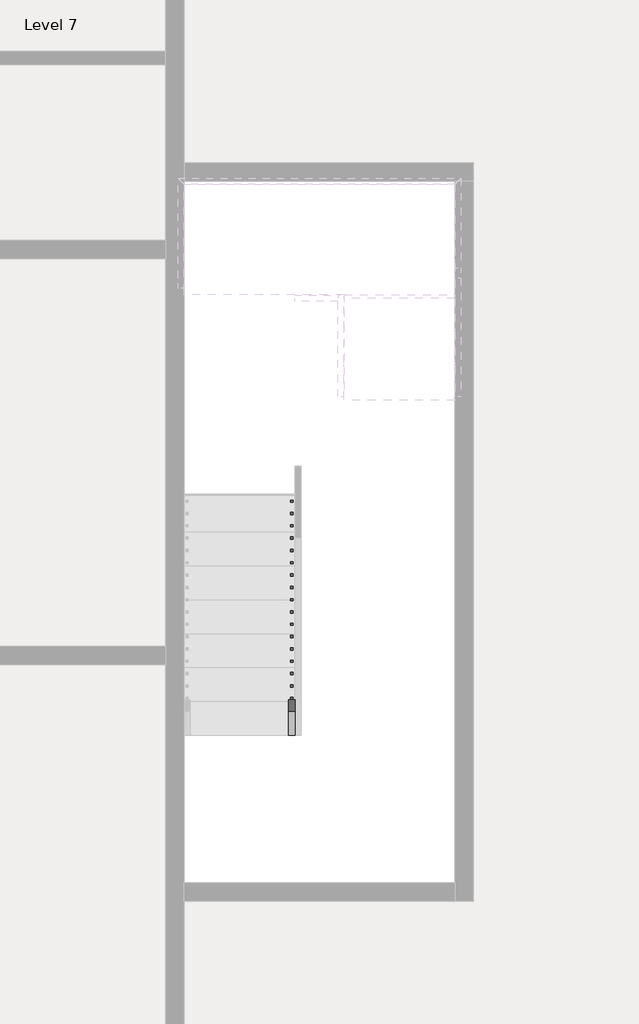
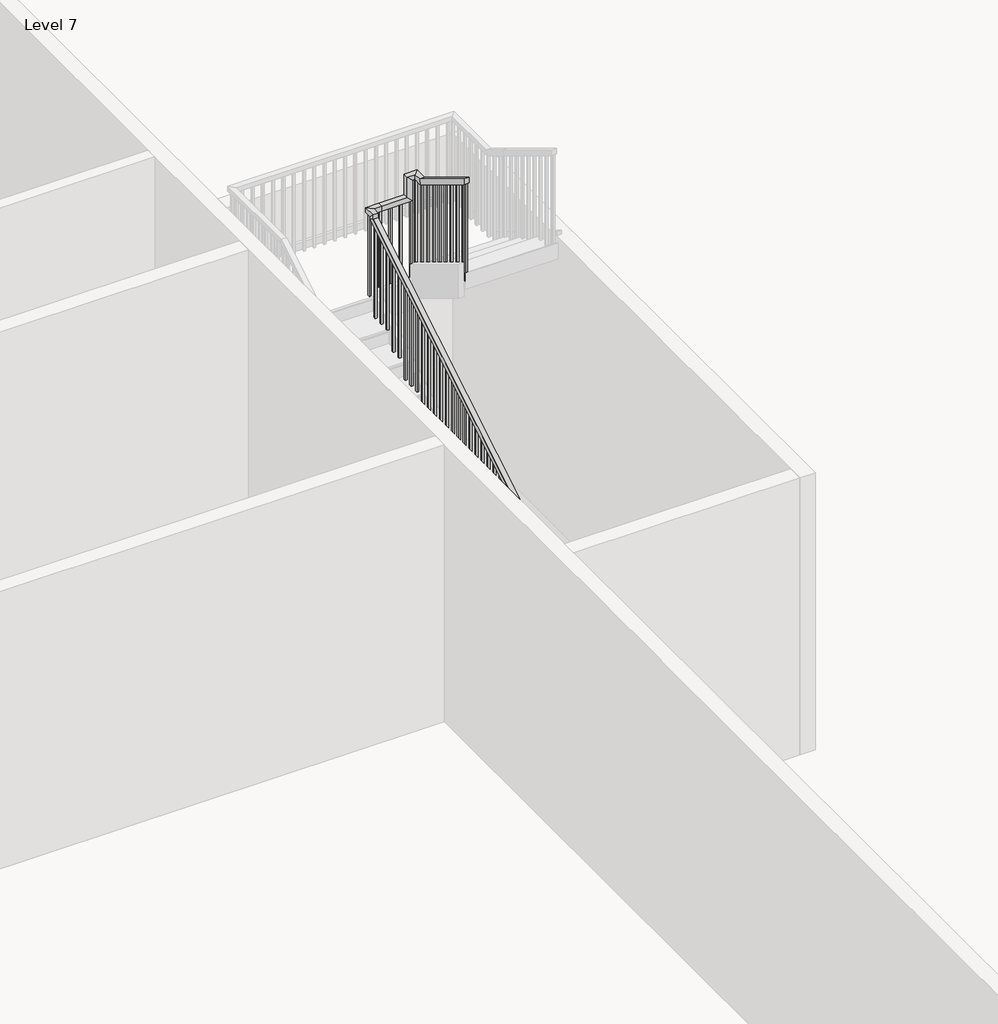
# One storey, part 5 of 8: 1 railing.
"""IFC4 building model written with IfcOpenShell, lengths in millimetres."""

from ifc_helpers import new_model, si_unit, frame, origin, place, context, project, spatial, polyline, outline, extrude, faceted_brep, element, save

model = new_model("IFC4")

# Units and contexts
model_context = context("Model", 3, world=origin())
ifc_project = project(units=[si_unit("LENGTHUNIT", "METRE", prefix="MILLI")], contexts=[model_context])

# Site, building, storey
site = spatial("IfcSite", under=ifc_project)
building = spatial("IfcBuilding", under=site)
storey = spatial("IfcBuildingStorey", under=building, Name="Level 7", Elevation=43522.6172466)

# Railing
placement = place(None, origin())
element("IfcRailing", 1, ObjectType="Handrail - Rectangular", at=placement, inside=storey, context=model_context, shape_type="SolidModel", body=[
    faceted_brep([(-2753.8415084, -23154.3851539, 44606.3505799), (-2753.8415084, -23154.3851539, 44546.9491197), (-2703.0415084, -23154.3851539, 44546.9491197), (-2703.0415084, -23154.3851539, 44606.3505799), (-2753.8415084, -19598.3851539, 46761.5020951), (-2753.8415084, -19547.5851539, 46732.8885136), (-2703.0415084, -19547.5851539, 46732.8885136), (-2703.0415084, -19598.3851539, 46761.5020951), (-2753.8415084, -19598.3851539, 46807.6839133), (-2753.8415084, -19547.5851539, 46756.8839133), (-2703.0415084, -19547.5851539, 46756.8839133), (-2703.0415084, -19598.3851539, 46807.6839133), (-2753.8415084, -19471.3851539, 46807.6839133), (-2753.8415084, -19471.3851539, 46756.8839133), (-2703.0415084, -19522.1851539, 46756.8839133), (-2703.0415084, -19522.1851539, 46807.6839133), (-2626.8415084, -19471.3851539, 46807.6839133), (-2626.8415084, -19471.3851539, 46756.8839133), (-2626.8415084, -19522.1851539, 46756.8839133), (-2626.8415084, -19522.1851539, 46807.6839133), (-2372.8415084, -19471.3851539, 46807.6839133), (-2322.0415084, -19471.3851539, 46756.8839133), (-2322.0415084, -19522.1851539, 46756.8839133), (-2372.8415084, -19522.1851539, 46807.6839133), (-2372.8415084, -19471.3851539, 47023.1990648), (-2322.0415084, -19471.3851539, 46972.3990648), (-2322.0415084, -19522.1851539, 46972.3990648), (-2372.8415084, -19522.1851539, 47023.1990648), (-2245.8415084, -19471.3851539, 47023.1990648), (-2245.8415084, -19471.3851539, 46972.3990648), (-2296.6415084, -19522.1851539, 46972.3990648), (-2296.6415084, -19522.1851539, 47023.1990648), (-2245.8415084, -19598.3851539, 47023.1990648), (-2245.8415084, -19612.5775633, 46972.3990648), (-2296.6415084, -19612.5775633, 46972.3990648), (-2296.6415084, -19598.3851539, 47023.1990648), (-2245.8415084, -20360.3851539, 47485.0172466), (-2296.6415084, -20360.3851539, 47485.0172466), (-2296.6415084, -20360.3851539, 47425.6157863), (-2245.8415084, -20360.3851539, 47425.6157863)], [[[0, 1, 2, 3]], [[1, 0, 4, 5]], [[2, 1, 5, 6]], [[3, 2, 6, 7]], [[0, 3, 7, 4]], [[5, 4, 8, 9]], [[6, 5, 9, 10]], [[7, 6, 10, 11]], [[4, 7, 11, 8]], [[9, 8, 12, 13]], [[10, 9, 13, 14]], [[11, 10, 14, 15]], [[8, 11, 15, 12]], [[13, 12, 16, 17]], [[14, 13, 17, 18]], [[15, 14, 18, 19]], [[12, 15, 19, 16]], [[17, 16, 20, 21]], [[18, 17, 21, 22]], [[19, 18, 22, 23]], [[16, 19, 23, 20]], [[21, 20, 24, 25]], [[22, 21, 25, 26]], [[23, 22, 26, 27]], [[20, 23, 27, 24]], [[25, 24, 28, 29]], [[26, 25, 29, 30]], [[27, 26, 30, 31]], [[24, 27, 31, 28]], [[29, 28, 32, 33]], [[30, 29, 33, 34]], [[31, 30, 34, 35]], [[28, 31, 35, 32]], [[36, 37, 38, 39]], [[33, 32, 36, 39]], [[34, 33, 39, 38]], [[35, 34, 38, 37]], [[32, 35, 37, 36]]]),
    extrude(outline(polyline([(-20319.1101539, 47400.6006348), (-20300.0601539, 47389.0551803), (-20300.0601539, 46401.2839133), (-20319.1101539, 46401.2839133), (-20319.1101539, 47400.6006348)])), frame((-2280.7665084, 0.0, 0.0), z_axis=(1.0, 0.0, 0.0), x_axis=(0.0, 1.0, 0.0)), (0.0, 0.0, 1.0), 19.05),
    extrude(outline(polyline([(-20217.5101539, 47339.0248773), (-20198.4601539, 47327.4794227), (-20198.4601539, 46401.2839133), (-20217.5101539, 46401.2839133), (-20217.5101539, 47339.0248773)])), frame((-2280.7665084, 0.0, 0.0), z_axis=(1.0, 0.0, 0.0), x_axis=(0.0, 1.0, 0.0)), (0.0, 0.0, 1.0), 19.05),
    extrude(outline(polyline([(-20115.9101539, 47277.4491197), (-20096.8601539, 47265.9036651), (-20096.8601539, 46401.2839133), (-20115.9101539, 46401.2839133), (-20115.9101539, 47277.4491197)])), frame((-2280.7665084, 0.0, 0.0), z_axis=(1.0, 0.0, 0.0), x_axis=(0.0, 1.0, 0.0)), (0.0, 0.0, 1.0), 19.05),
    extrude(outline(polyline([(-20014.3101539, 47215.8733621), (-19995.2601539, 47204.3279076), (-19995.2601539, 46231.9505799), (-20014.3101539, 46231.9505799), (-20014.3101539, 47215.8733621)])), frame((-2280.7665084, 0.0, 0.0), z_axis=(1.0, 0.0, 0.0), x_axis=(0.0, 1.0, 0.0)), (0.0, 0.0, 1.0), 19.05),
    extrude(outline(polyline([(-19912.7101539, 47154.2976045), (-19893.6601539, 47142.75215), (-19893.6601539, 46231.9505799), (-19912.7101539, 46231.9505799), (-19912.7101539, 47154.2976045)])), frame((-2280.7665084, 0.0, 0.0), z_axis=(1.0, 0.0, 0.0), x_axis=(0.0, 1.0, 0.0)), (0.0, 0.0, 1.0), 19.05),
    extrude(outline(polyline([(-19811.1101539, 47092.721847), (-19792.0601539, 47081.1763924), (-19792.0601539, 46231.9505799), (-19811.1101539, 46231.9505799), (-19811.1101539, 47092.721847)])), frame((-2280.7665084, 0.0, 0.0), z_axis=(1.0, 0.0, 0.0), x_axis=(0.0, 1.0, 0.0)), (0.0, 0.0, 1.0), 19.05),
    extrude(outline(polyline([(-19709.5101539, 47031.1460894), (-19690.4601539, 47019.6006348), (-19690.4601539, 46062.6172466), (-19709.5101539, 46062.6172466), (-19709.5101539, 47031.1460894)])), frame((-2280.7665084, 0.0, 0.0), z_axis=(1.0, 0.0, 0.0), x_axis=(0.0, 1.0, 0.0)), (0.0, 0.0, 1.0), 19.05),
    extrude(outline(polyline([(-19607.9101539, 46969.5703318), (-19588.8601539, 46958.0248773), (-19588.8601539, 46062.6172466), (-19607.9101539, 46062.6172466), (-19607.9101539, 46969.5703318)])), frame((-2280.7665084, 0.0, 0.0), z_axis=(1.0, 0.0, 0.0), x_axis=(0.0, 1.0, 0.0)), (0.0, 0.0, 1.0), 19.05),
    extrude(outline(polyline([(-2331.5665084, -19506.3101539), (-2331.5665084, -19487.2601539), (-2312.5165084, -19487.2601539), (-2312.5165084, -19506.3101539), (-2331.5665084, -19506.3101539)])), frame((0.0, 0.0, 45893.2839133), z_axis=(0.0, 0.0, 1.0), x_axis=(1.0, 0.0, 0.0)), (0.0, 0.0, 1.0), 1079.1151515),
    extrude(outline(polyline([(-2433.1665084, -19506.3101539), (-2433.1665084, -19487.2601539), (-2414.1165084, -19487.2601539), (-2414.1165084, -19506.3101539), (-2433.1665084, -19506.3101539)])), frame((0.0, 0.0, 45893.2839133), z_axis=(0.0, 0.0, 1.0), x_axis=(1.0, 0.0, 0.0)), (0.0, 0.0, 1.0), 863.6),
    extrude(outline(polyline([(-2534.7665084, -19506.3101539), (-2534.7665084, -19487.2601539), (-2515.7165084, -19487.2601539), (-2515.7165084, -19506.3101539), (-2534.7665084, -19506.3101539)])), frame((0.0, 0.0, 45893.2839133), z_axis=(0.0, 0.0, 1.0), x_axis=(1.0, 0.0, 0.0)), (0.0, 0.0, 1.0), 863.6),
    extrude(outline(polyline([(-2636.3665084, -19506.3101539), (-2636.3665084, -19487.2601539), (-2617.3165084, -19487.2601539), (-2617.3165084, -19506.3101539), (-2636.3665084, -19506.3101539)])), frame((0.0, 0.0, 45893.2839133), z_axis=(0.0, 0.0, 1.0), x_axis=(1.0, 0.0, 0.0)), (0.0, 0.0, 1.0), 863.6),
    extrude(outline(polyline([(-19607.9101539, 46696.3279076), (-19588.8601539, 46707.8733621), (-19588.8601539, 45723.9505799), (-19607.9101539, 45723.9505799), (-19607.9101539, 46696.3279076)])), frame((-2737.9665084, 0.0, 0.0), z_axis=(1.0, 0.0, 0.0), x_axis=(0.0, 1.0, 0.0)), (0.0, 0.0, 1.0), 19.05),
    extrude(outline(polyline([(-19709.5101539, 46634.75215), (-19690.4601539, 46646.2976045), (-19690.4601539, 45723.9505799), (-19709.5101539, 45723.9505799), (-19709.5101539, 46634.75215)])), frame((-2737.9665084, 0.0, 0.0), z_axis=(1.0, 0.0, 0.0), x_axis=(0.0, 1.0, 0.0)), (0.0, 0.0, 1.0), 19.05),
    extrude(outline(polyline([(-19811.1101539, 46573.1763924), (-19792.0601539, 46584.721847), (-19792.0601539, 45723.9505799), (-19811.1101539, 45723.9505799), (-19811.1101539, 46573.1763924)])), frame((-2737.9665084, 0.0, 0.0), z_axis=(1.0, 0.0, 0.0), x_axis=(0.0, 1.0, 0.0)), (0.0, 0.0, 1.0), 19.05),
    extrude(outline(polyline([(-19912.7101539, 46511.6006348), (-19893.6601539, 46523.1460894), (-19893.6601539, 45554.6172466), (-19912.7101539, 45554.6172466), (-19912.7101539, 46511.6006348)])), frame((-2737.9665084, 0.0, 0.0), z_axis=(1.0, 0.0, 0.0), x_axis=(0.0, 1.0, 0.0)), (0.0, 0.0, 1.0), 19.05),
    extrude(outline(polyline([(-20014.3101539, 46450.0248773), (-19995.2601539, 46461.5703318), (-19995.2601539, 45554.6172466), (-20014.3101539, 45554.6172466), (-20014.3101539, 46450.0248773)])), frame((-2737.9665084, 0.0, 0.0), z_axis=(1.0, 0.0, 0.0), x_axis=(0.0, 1.0, 0.0)), (0.0, 0.0, 1.0), 19.05),
    extrude(outline(polyline([(-20115.9101539, 46388.4491197), (-20096.8601539, 46399.9945742), (-20096.8601539, 45385.2839133), (-20115.9101539, 45385.2839133), (-20115.9101539, 46388.4491197)])), frame((-2737.9665084, 0.0, 0.0), z_axis=(1.0, 0.0, 0.0), x_axis=(0.0, 1.0, 0.0)), (0.0, 0.0, 1.0), 19.05),
    extrude(outline(polyline([(-20217.5101539, 46326.8733621), (-20198.4601539, 46338.4188166), (-20198.4601539, 45385.2839133), (-20217.5101539, 45385.2839133), (-20217.5101539, 46326.8733621)])), frame((-2737.9665084, 0.0, 0.0), z_axis=(1.0, 0.0, 0.0), x_axis=(0.0, 1.0, 0.0)), (0.0, 0.0, 1.0), 19.05),
    extrude(outline(polyline([(-20319.1101539, 46265.2976045), (-20300.0601539, 46276.8430591), (-20300.0601539, 45385.2839133), (-20319.1101539, 45385.2839133), (-20319.1101539, 46265.2976045)])), frame((-2737.9665084, 0.0, 0.0), z_axis=(1.0, 0.0, 0.0), x_axis=(0.0, 1.0, 0.0)), (0.0, 0.0, 1.0), 19.05),
    extrude(outline(polyline([(-20420.7101539, 46203.721847), (-20401.6601539, 46215.2673015), (-20401.6601539, 45215.9505799), (-20420.7101539, 45215.9505799), (-20420.7101539, 46203.721847)])), frame((-2737.9665084, 0.0, 0.0), z_axis=(1.0, 0.0, 0.0), x_axis=(0.0, 1.0, 0.0)), (0.0, 0.0, 1.0), 19.05),
    extrude(outline(polyline([(-20522.3101539, 46142.1460894), (-20503.2601539, 46153.6915439), (-20503.2601539, 45215.9505799), (-20522.3101539, 45215.9505799), (-20522.3101539, 46142.1460894)])), frame((-2737.9665084, 0.0, 0.0), z_axis=(1.0, 0.0, 0.0), x_axis=(0.0, 1.0, 0.0)), (0.0, 0.0, 1.0), 19.05),
    extrude(outline(polyline([(-20623.9101539, 46080.5703318), (-20604.8601539, 46092.1157863), (-20604.8601539, 45215.9505799), (-20623.9101539, 45215.9505799), (-20623.9101539, 46080.5703318)])), frame((-2737.9665084, 0.0, 0.0), z_axis=(1.0, 0.0, 0.0), x_axis=(0.0, 1.0, 0.0)), (0.0, 0.0, 1.0), 19.05),
    extrude(outline(polyline([(-20725.5101539, 46018.9945742), (-20706.4601539, 46030.5400288), (-20706.4601539, 45046.6172466), (-20725.5101539, 45046.6172466), (-20725.5101539, 46018.9945742)])), frame((-2737.9665084, 0.0, 0.0), z_axis=(1.0, 0.0, 0.0), x_axis=(0.0, 1.0, 0.0)), (0.0, 0.0, 1.0), 19.05),
    extrude(outline(polyline([(-20827.1101539, 45957.4188166), (-20808.0601539, 45968.9642712), (-20808.0601539, 45046.6172466), (-20827.1101539, 45046.6172466), (-20827.1101539, 45957.4188166)])), frame((-2737.9665084, 0.0, 0.0), z_axis=(1.0, 0.0, 0.0), x_axis=(0.0, 1.0, 0.0)), (0.0, 0.0, 1.0), 19.05),
    extrude(outline(polyline([(-20928.7101539, 45895.8430591), (-20909.6601539, 45907.3885136), (-20909.6601539, 45046.6172466), (-20928.7101539, 45046.6172466), (-20928.7101539, 45895.8430591)])), frame((-2737.9665084, 0.0, 0.0), z_axis=(1.0, 0.0, 0.0), x_axis=(0.0, 1.0, 0.0)), (0.0, 0.0, 1.0), 19.05),
    extrude(outline(polyline([(-21030.3101539, 45834.2673015), (-21011.2601539, 45845.812756), (-21011.2601539, 44877.2839133), (-21030.3101539, 44877.2839133), (-21030.3101539, 45834.2673015)])), frame((-2737.9665084, 0.0, 0.0), z_axis=(1.0, 0.0, 0.0), x_axis=(0.0, 1.0, 0.0)), (0.0, 0.0, 1.0), 19.05),
    extrude(outline(polyline([(-21131.9101539, 45772.6915439), (-21112.8601539, 45784.2369985), (-21112.8601539, 44877.2839133), (-21131.9101539, 44877.2839133), (-21131.9101539, 45772.6915439)])), frame((-2737.9665084, 0.0, 0.0), z_axis=(1.0, 0.0, 0.0), x_axis=(0.0, 1.0, 0.0)), (0.0, 0.0, 1.0), 19.05),
    extrude(outline(polyline([(-21233.5101539, 45711.1157863), (-21214.4601539, 45722.6612409), (-21214.4601539, 44707.9505799), (-21233.5101539, 44707.9505799), (-21233.5101539, 45711.1157863)])), frame((-2737.9665084, 0.0, 0.0), z_axis=(1.0, 0.0, 0.0), x_axis=(0.0, 1.0, 0.0)), (0.0, 0.0, 1.0), 19.05),
    extrude(outline(polyline([(-21335.1101539, 45649.5400288), (-21316.0601539, 45661.0854833), (-21316.0601539, 44707.9505799), (-21335.1101539, 44707.9505799), (-21335.1101539, 45649.5400288)])), frame((-2737.9665084, 0.0, 0.0), z_axis=(1.0, 0.0, 0.0), x_axis=(0.0, 1.0, 0.0)), (0.0, 0.0, 1.0), 19.05),
    extrude(outline(polyline([(-21436.7101539, 45587.9642712), (-21417.6601539, 45599.5097257), (-21417.6601539, 44707.9505799), (-21436.7101539, 44707.9505799), (-21436.7101539, 45587.9642712)])), frame((-2737.9665084, 0.0, 0.0), z_axis=(1.0, 0.0, 0.0), x_axis=(0.0, 1.0, 0.0)), (0.0, 0.0, 1.0), 19.05),
    extrude(outline(polyline([(-21538.3101539, 45526.3885136), (-21519.2601539, 45537.9339682), (-21519.2601539, 44538.6172466), (-21538.3101539, 44538.6172466), (-21538.3101539, 45526.3885136)])), frame((-2737.9665084, 0.0, 0.0), z_axis=(1.0, 0.0, 0.0), x_axis=(0.0, 1.0, 0.0)), (0.0, 0.0, 1.0), 19.05),
    extrude(outline(polyline([(-21639.9101539, 45464.812756), (-21620.8601539, 45476.3582106), (-21620.8601539, 44538.6172466), (-21639.9101539, 44538.6172466), (-21639.9101539, 45464.812756)])), frame((-2737.9665084, 0.0, 0.0), z_axis=(1.0, 0.0, 0.0), x_axis=(0.0, 1.0, 0.0)), (0.0, 0.0, 1.0), 19.05),
    extrude(outline(polyline([(-21741.5101539, 45403.2369985), (-21722.4601539, 45414.782453), (-21722.4601539, 44538.6172466), (-21741.5101539, 44538.6172466), (-21741.5101539, 45403.2369985)])), frame((-2737.9665084, 0.0, 0.0), z_axis=(1.0, 0.0, 0.0), x_axis=(0.0, 1.0, 0.0)), (0.0, 0.0, 1.0), 19.05),
    extrude(outline(polyline([(-21843.1101539, 45341.6612409), (-21824.0601539, 45353.2066954), (-21824.0601539, 44369.2839133), (-21843.1101539, 44369.2839133), (-21843.1101539, 45341.6612409)])), frame((-2737.9665084, 0.0, 0.0), z_axis=(1.0, 0.0, 0.0), x_axis=(0.0, 1.0, 0.0)), (0.0, 0.0, 1.0), 19.05),
    extrude(outline(polyline([(-21944.7101539, 45280.0854833), (-21925.6601539, 45291.6309379), (-21925.6601539, 44369.2839133), (-21944.7101539, 44369.2839133), (-21944.7101539, 45280.0854833)])), frame((-2737.9665084, 0.0, 0.0), z_axis=(1.0, 0.0, 0.0), x_axis=(0.0, 1.0, 0.0)), (0.0, 0.0, 1.0), 19.05),
    extrude(outline(polyline([(-22046.3101539, 45218.5097257), (-22027.2601539, 45230.0551803), (-22027.2601539, 44369.2839133), (-22046.3101539, 44369.2839133), (-22046.3101539, 45218.5097257)])), frame((-2737.9665084, 0.0, 0.0), z_axis=(1.0, 0.0, 0.0), x_axis=(0.0, 1.0, 0.0)), (0.0, 0.0, 1.0), 19.05),
    extrude(outline(polyline([(-22147.9101539, 45156.9339682), (-22128.8601539, 45168.4794227), (-22128.8601539, 44199.9505799), (-22147.9101539, 44199.9505799), (-22147.9101539, 45156.9339682)])), frame((-2737.9665084, 0.0, 0.0), z_axis=(1.0, 0.0, 0.0), x_axis=(0.0, 1.0, 0.0)), (0.0, 0.0, 1.0), 19.05),
    extrude(outline(polyline([(-22249.5101539, 45095.3582106), (-22230.4601539, 45106.9036651), (-22230.4601539, 44199.9505799), (-22249.5101539, 44199.9505799), (-22249.5101539, 45095.3582106)])), frame((-2737.9665084, 0.0, 0.0), z_axis=(1.0, 0.0, 0.0), x_axis=(0.0, 1.0, 0.0)), (0.0, 0.0, 1.0), 19.05),
    extrude(outline(polyline([(-22351.1101539, 45033.782453), (-22332.0601539, 45045.3279076), (-22332.0601539, 44030.6172466), (-22351.1101539, 44030.6172466), (-22351.1101539, 45033.782453)])), frame((-2737.9665084, 0.0, 0.0), z_axis=(1.0, 0.0, 0.0), x_axis=(0.0, 1.0, 0.0)), (0.0, 0.0, 1.0), 19.05),
    extrude(outline(polyline([(-22452.7101539, 44972.2066954), (-22433.6601539, 44983.75215), (-22433.6601539, 44030.6172466), (-22452.7101539, 44030.6172466), (-22452.7101539, 44972.2066954)])), frame((-2737.9665084, 0.0, 0.0), z_axis=(1.0, 0.0, 0.0), x_axis=(0.0, 1.0, 0.0)), (0.0, 0.0, 1.0), 19.05),
    extrude(outline(polyline([(-22554.3101539, 44910.6309379), (-22535.2601539, 44922.1763924), (-22535.2601539, 44030.6172466), (-22554.3101539, 44030.6172466), (-22554.3101539, 44910.6309379)])), frame((-2737.9665084, 0.0, 0.0), z_axis=(1.0, 0.0, 0.0), x_axis=(0.0, 1.0, 0.0)), (0.0, 0.0, 1.0), 19.05),
    extrude(outline(polyline([(-22655.9101539, 44849.0551803), (-22636.8601539, 44860.6006348), (-22636.8601539, 43861.2839133), (-22655.9101539, 43861.2839133), (-22655.9101539, 44849.0551803)])), frame((-2737.9665084, 0.0, 0.0), z_axis=(1.0, 0.0, 0.0), x_axis=(0.0, 1.0, 0.0)), (0.0, 0.0, 1.0), 19.05),
    extrude(outline(polyline([(-22757.5101539, 44787.4794227), (-22738.4601539, 44799.0248773), (-22738.4601539, 43861.2839133), (-22757.5101539, 43861.2839133), (-22757.5101539, 44787.4794227)])), frame((-2737.9665084, 0.0, 0.0), z_axis=(1.0, 0.0, 0.0), x_axis=(0.0, 1.0, 0.0)), (0.0, 0.0, 1.0), 19.05),
    extrude(outline(polyline([(-22859.1101539, 44725.9036651), (-22840.0601539, 44737.4491197), (-22840.0601539, 43861.2839133), (-22859.1101539, 43861.2839133), (-22859.1101539, 44725.9036651)])), frame((-2737.9665084, 0.0, 0.0), z_axis=(1.0, 0.0, 0.0), x_axis=(0.0, 1.0, 0.0)), (0.0, 0.0, 1.0), 19.05),
    extrude(outline(polyline([(-22960.7101539, 44664.3279076), (-22941.6601539, 44675.8733621), (-22941.6601539, 43691.9505799), (-22960.7101539, 43691.9505799), (-22960.7101539, 44664.3279076)])), frame((-2737.9665084, 0.0, 0.0), z_axis=(1.0, 0.0, 0.0), x_axis=(0.0, 1.0, 0.0)), (0.0, 0.0, 1.0), 19.05),
    extrude(outline(polyline([(-23062.3101539, 44602.75215), (-23043.2601539, 44614.2976045), (-23043.2601539, 43691.9505799), (-23062.3101539, 43691.9505799), (-23062.3101539, 44602.75215)])), frame((-2737.9665084, 0.0, 0.0), z_axis=(1.0, 0.0, 0.0), x_axis=(0.0, 1.0, 0.0)), (0.0, 0.0, 1.0), 19.05),
    extrude(outline(polyline([(-2280.7665084, -19506.3101539), (-2280.7665084, -19487.2601539), (-2261.7165084, -19487.2601539), (-2261.7165084, -19506.3101539), (-2280.7665084, -19506.3101539)])), frame((0.0, 0.0, 45893.2839133), z_axis=(0.0, 0.0, 1.0), x_axis=(1.0, 0.0, 0.0)), (0.0, 0.0, 1.0), 1079.1151515),
    extrude(outline(polyline([(-2718.9165084, -19506.3101539), (-2737.9665084, -19506.3101539), (-2737.9665084, -19487.2601539), (-2718.9165084, -19487.2601539), (-2718.9165084, -19506.3101539)])), frame((0.0, 0.0, 45893.2839133), z_axis=(0.0, 0.0, 1.0), x_axis=(1.0, 0.0, 0.0)), (0.0, 0.0, 1.0), 863.6),
    extrude(outline(polyline([(-20360.3851539, 47425.6157863), (-20341.3351539, 47414.0703318), (-20341.3351539, 46401.2839133), (-20360.3851539, 46401.2839133), (-20360.3851539, 47425.6157863)])), frame((-2280.7665084, 0.0, 0.0), z_axis=(1.0, 0.0, 0.0), x_axis=(0.0, 1.0, 0.0)), (0.0, 0.0, 1.0), 19.05),
    extrude(outline(polyline([(-23154.3851539, 44546.9491197), (-23135.3351539, 44558.4945742), (-23135.3351539, 43691.9505799), (-23154.3851539, 43691.9505799), (-23154.3851539, 44546.9491197)])), frame((-2737.9665084, 0.0, 0.0), z_axis=(1.0, 0.0, 0.0), x_axis=(0.0, 1.0, 0.0)), (0.0, 0.0, 1.0), 19.05),
])

save(model, "model.ifc")

# Revit data of these elements
# Type "Handrail - Rectangular"
#   Assembly Code = "C2010400"
#   built-in parameter 1008612 = 0.0416667 (stored number, unit not read)
#   built-in parameter 1008611 = 0.0416667 (stored number, unit not read)
#   built-in parameter 1008609 = 0.333333 (stored number, unit not read)
#   built-in parameter 1008604 = 0.166667 (stored number, unit not read)
#   built-in parameter 1008603 = 0.166667 (stored number, unit not read)
#   Railing Height = 3' - 0"
#   built-in parameter 1008630 = 2
#   built-in parameter 1008610 = 2
#   built-in parameter 1008618 = Baluster - Square : 3/4"
# Element 1 (IfcRailing, "Handrail - Rectangular")
#   Phase Created = New Construction
